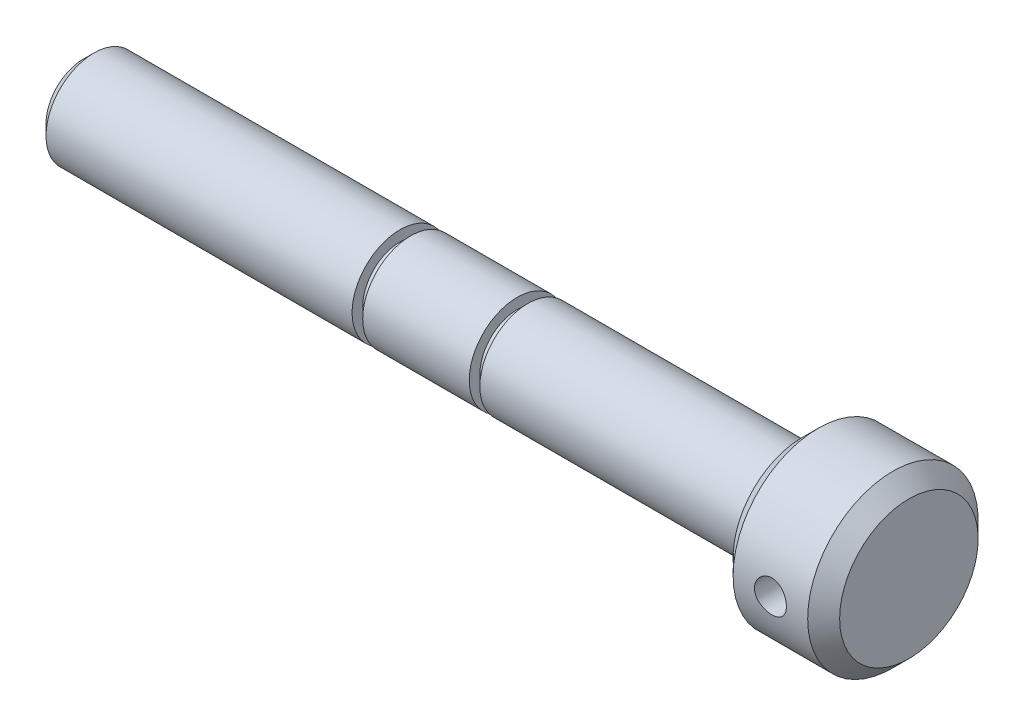
from build123d import *

# Parameters (mm, degrees)
HEAD_CHAMFER_3MM_SIZE      = 3
EDGE_CHAMFER_2MM_SIZE      = 2
HEAD_CROSS_HOLE_DEPTH      = 157.642906
HEAD_CROSS_HOLE_DEPTH_BACK = 157.642906
CROSS_HOLE_SKETCH_R        = 3


with BuildPart() as part:
    # Bolt Profile Sketch → Bolt Body Revolve (revolve)
    with BuildSketch(Plane.XY, mode=Mode.PRIVATE) as bolt_body_revolve_sk:
        Polygon((155, 0), (155, 16), (135, 16), (135, 9), (83.46, 9), (83.46, 7), (81.46, 7), (81.46, 9), (61.46, 9), (61.46, 7), (59.46, 7), (59.46, 9), (0, 9), (0, 0), align=None)
    revolve(bolt_body_revolve_sk.sketch.rotate(Axis((0, 0, 0), (1, 0, 0)), 90), axis=Axis((0, 0, 0), (1, 0, 0)))

    # Head Chamfer 3mm
    head_chamfer_3mm_edges = [part.edges().sort_by_distance(p)[0] for p in [
        (135, 0, -16),
        (155, 0, -16),
    ]]
    chamfer(head_chamfer_3mm_edges, length=HEAD_CHAMFER_3MM_SIZE)

    # Edge Chamfer 2mm
    edge_chamfer_2mm_edges = [part.edges().sort_by_distance(p)[0] for p in [
        (0, 0, -9),
    ]]
    chamfer(edge_chamfer_2mm_edges, length=EDGE_CHAMFER_2MM_SIZE)

    # Cross Hole Sketch → Head Cross Hole (cut, two sides: drawn at the far end of the back side and taken through both)
    with BuildSketch(Plane.XY.offset(-HEAD_CROSS_HOLE_DEPTH_BACK)):
        with Locations((145, 0)):
            Circle(CROSS_HOLE_SKETCH_R)
    extrude(amount=HEAD_CROSS_HOLE_DEPTH + HEAD_CROSS_HOLE_DEPTH_BACK, mode=Mode.SUBTRACT)


solid = part.part
